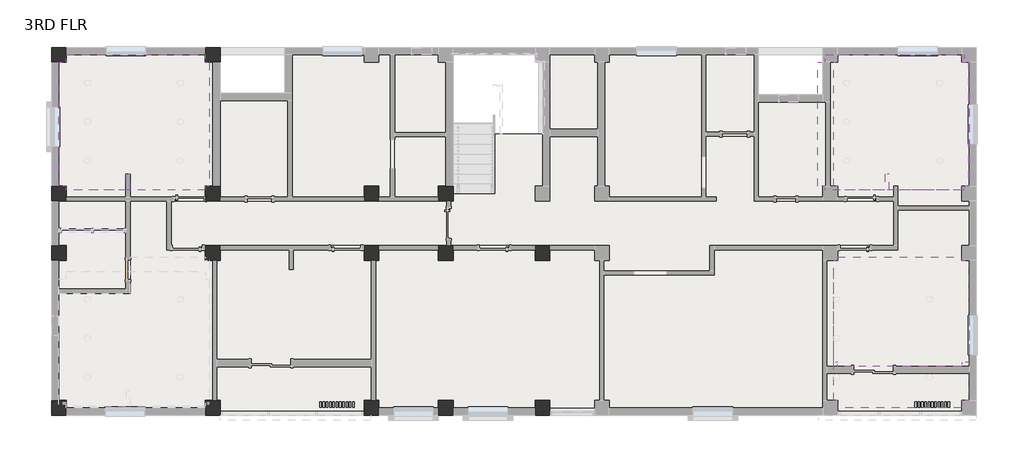
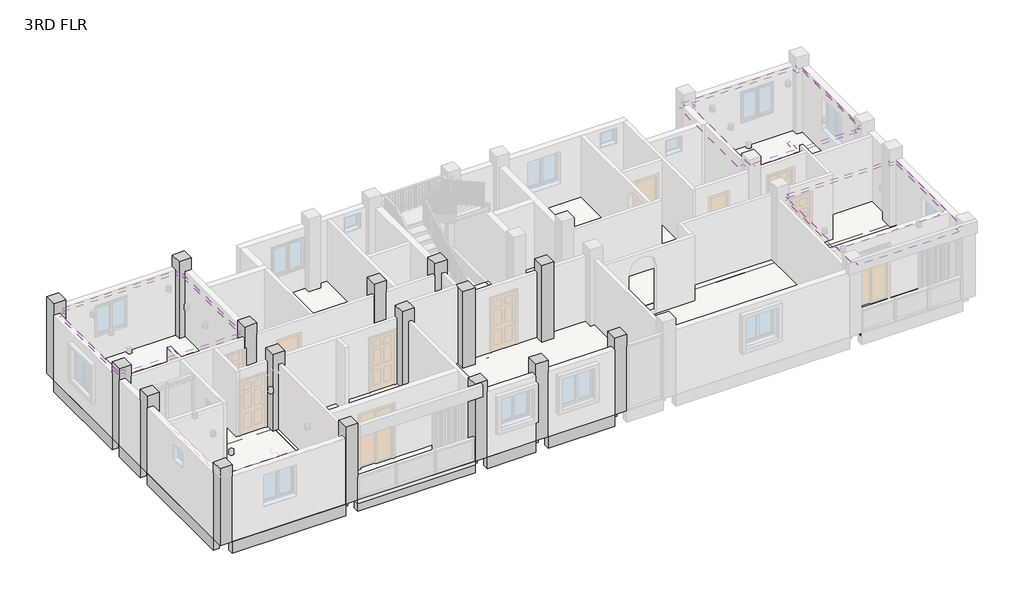
# One storey, part 3 of 5: 23 beams, 16 columns, 6 coverings, 3 slabs.
"""IFC4 building model written with IfcOpenShell, lengths in millimetres."""

from ifc_helpers import new_model, si_unit, point, frame, frame_2d, origin, place, context, project, spatial, polyline, circle_curve, trimmed, segment, composite_curve, outline, extrude, element, save

model = new_model("IFC4")

# Units and contexts
model_context = context("Model", 3, world=origin())
ifc_project = project(units=[si_unit("LENGTHUNIT", "METRE", prefix="MILLI")], contexts=[model_context])

# Site, building, storey
site = spatial("IfcSite", under=ifc_project)
building = spatial("IfcBuilding", under=site)
storey = spatial("IfcBuildingStorey", under=building, Name="3RD FLR", Elevation=9448.8)

# Beams
placement = place(None, origin())
element("IfcBeam", 1, ObjectType="Concrete-Rectangular Beam : 9\" X 18\" BEAM", at=placement, inside=storey, context=model_context, shape_type="SweptSolid", body=[
    extrude(outline(polyline([(-10649.5456086, -10887.8679047), (-10649.5456086, -11116.4679047), (-14916.7456086, -11116.4679047), (-14916.7456086, -10887.8679047), (-10649.5456086, -10887.8679047)])), frame((0.0, 0.0, 8991.6), z_axis=(0.0, 0.0, 1.0), x_axis=(1.0, 0.0, 0.0)), (0.0, 0.0, 1.0), 457.2),
])
element("IfcBeam", 2, ObjectType="Concrete-Rectangular Beam : 9\" X 18\" BEAM", at=placement, inside=storey, context=model_context, shape_type="SweptSolid", body=[
    extrude(outline(polyline([(-5772.7456086, -10887.8679047), (-5772.7456086, -11116.4679047), (-10192.3456086, -11116.4679047), (-10192.3456086, -10887.8679047), (-5772.7456086, -10887.8679047)])), frame((0.0, 0.0, 8991.6), z_axis=(0.0, 0.0, 1.0), x_axis=(1.0, 0.0, 0.0)), (0.0, 0.0, 1.0), 457.2),
])
element("IfcBeam", 3, ObjectType="Concrete-Rectangular Beam : 9\" X 18\" BEAM", at=placement, inside=storey, context=model_context, shape_type="SweptSolid", body=[
    extrude(outline(polyline([(-3486.7456086, -10887.8679047), (-3486.7456086, -11116.4679047), (-5315.5456086, -11116.4679047), (-5315.5456086, -10887.8679047), (-3486.7456086, -10887.8679047)])), frame((0.0, 0.0, 8991.6), z_axis=(0.0, 0.0, 1.0), x_axis=(1.0, 0.0, 0.0)), (0.0, 0.0, 1.0), 457.2),
])
element("IfcBeam", 4, ObjectType="Concrete-Rectangular Beam : 9\" X 18\" BEAM", at=placement, inside=storey, context=model_context, shape_type="SweptSolid", body=[
    extrude(outline(polyline([(-518.4083398, -10887.8679047), (-518.4083398, -11116.4679047), (-3029.5456086, -11116.4679047), (-3029.5456086, -10887.8679047), (-518.4083398, -10887.8679047)])), frame((0.0, 0.0, 8991.6), z_axis=(0.0, 0.0, 1.0), x_axis=(1.0, 0.0, 0.0)), (0.0, 0.0, 1.0), 457.2),
])
element("IfcBeam", 5, ObjectType="Concrete-Rectangular Beam : 9\" X 18\" BEAM", at=placement, inside=storey, context=model_context, shape_type="SweptSolid", body=[
    extrude(outline(polyline([(-15145.3456086, -4072.3794704), (-15373.9456086, -4072.3794704), (-15373.9456086, -262.3794704), (-15145.3456086, -262.3794704), (-15145.3456086, -4072.3794704)])), frame((0.0, 0.0, 8991.6), z_axis=(0.0, 0.0, 1.0), x_axis=(1.0, 0.0, 0.0)), (0.0, 0.0, 1.0), 457.2),
])
element("IfcBeam", 6, ObjectType="Concrete-Rectangular Beam : 9\" X 18\" BEAM", at=placement, inside=storey, context=model_context, shape_type="SweptSolid", body=[
    extrude(outline(polyline([(-15145.3456086, -5901.1794704), (-15373.9456086, -5901.1794704), (-15373.9456086, -4529.5794704), (-15145.3456086, -4529.5794704), (-15145.3456086, -5901.1794704)])), frame((0.0, 0.0, 8991.6), z_axis=(0.0, 0.0, 1.0), x_axis=(1.0, 0.0, 0.0)), (0.0, 0.0, 1.0), 457.2),
])
element("IfcBeam", 7, ObjectType="Concrete-Rectangular Beam : 9\" X 18\" BEAM", at=placement, inside=storey, context=model_context, shape_type="SweptSolid", body=[
    extrude(outline(polyline([(-15145.3456086, -10659.2679047), (-15373.9456086, -10659.2679047), (-15373.9456086, -6358.3794704), (-15145.3456086, -6358.3794704), (-15145.3456086, -10659.2679047)])), frame((0.0, 0.0, 8991.6), z_axis=(0.0, 0.0, 1.0), x_axis=(1.0, 0.0, 0.0)), (0.0, 0.0, 1.0), 457.2),
])
element("IfcBeam", 8, ObjectType="Concrete-Rectangular Beam : 9\" X 18\" BEAM", at=placement, inside=storey, context=model_context, shape_type="SweptSolid", body=[
    extrude(outline(polyline([(-10649.5456086, -4186.6794704), (-10649.5456086, -4415.2794704), (-14916.7456086, -4415.2794704), (-14916.7456086, -4186.6794704), (-10649.5456086, -4186.6794704)])), frame((0.0, 0.0, 8991.6), z_axis=(0.0, 0.0, 1.0), x_axis=(1.0, 0.0, 0.0)), (0.0, 0.0, 1.0), 457.2),
])
element("IfcBeam", 9, ObjectType="Concrete-Rectangular Beam : 9\" X 18\" BEAM", at=placement, inside=storey, context=model_context, shape_type="SweptSolid", body=[
    extrude(outline(polyline([(-5772.7456086, -4186.6794704), (-5772.7456086, -4415.2794704), (-10192.3456086, -4415.2794704), (-10192.3456086, -4186.6794704), (-5772.7456086, -4186.6794704)])), frame((0.0, 0.0, 8991.6), z_axis=(0.0, 0.0, 1.0), x_axis=(1.0, 0.0, 0.0)), (0.0, 0.0, 1.0), 457.2),
])
element("IfcBeam", 10, ObjectType="Concrete-Rectangular Beam : 9\" X 18\" BEAM", at=placement, inside=storey, context=model_context, shape_type="SweptSolid", body=[
    extrude(outline(polyline([(-3486.7456086, -4186.6794704), (-3486.7456086, -4415.2794704), (-5315.5456086, -4415.2794704), (-5315.5456086, -4186.6794704), (-3486.7456086, -4186.6794704)])), frame((0.0, 0.0, 8991.6), z_axis=(0.0, 0.0, 1.0), x_axis=(1.0, 0.0, 0.0)), (0.0, 0.0, 1.0), 457.2),
])
element("IfcBeam", 11, ObjectType="Concrete-Rectangular Beam : 9\" X 18\" BEAM", at=placement, inside=storey, context=model_context, shape_type="SweptSolid", body=[
    extrude(outline(polyline([(-10306.6456086, -4072.3794704), (-10535.2456086, -4072.3794704), (-10535.2456086, -262.3794704), (-10306.6456086, -262.3794704), (-10306.6456086, -4072.3794704)])), frame((0.0, 0.0, 8991.6), z_axis=(0.0, 0.0, 1.0), x_axis=(1.0, 0.0, 0.0)), (0.0, 0.0, 1.0), 457.2),
])
element("IfcBeam", 12, ObjectType="Concrete-Rectangular Beam : 9\" X 18\" BEAM", at=placement, inside=storey, context=model_context, shape_type="SweptSolid", body=[
    extrude(outline(polyline([(-10649.5456086, -6015.4794704), (-10649.5456086, -6244.0794704), (-14916.7456086, -6244.0794704), (-14916.7456086, -6015.4794704), (-10649.5456086, -6015.4794704)])), frame((0.0, 0.0, 8991.6), z_axis=(0.0, 0.0, 1.0), x_axis=(1.0, 0.0, 0.0)), (0.0, 0.0, 1.0), 457.2),
])
element("IfcBeam", 13, ObjectType="Concrete-Rectangular Beam : 9\" X 18\" BEAM", at=placement, inside=storey, context=model_context, shape_type="SweptSolid", body=[
    extrude(outline(polyline([(-5772.7456086, -6015.4794704), (-5772.7456086, -6244.0794704), (-10192.3456086, -6244.0794704), (-10192.3456086, -6015.4794704), (-5772.7456086, -6015.4794704)])), frame((0.0, 0.0, 8991.6), z_axis=(0.0, 0.0, 1.0), x_axis=(1.0, 0.0, 0.0)), (0.0, 0.0, 1.0), 457.2),
])
element("IfcBeam", 14, ObjectType="Concrete-Rectangular Beam : 9\" X 18\" BEAM", at=placement, inside=storey, context=model_context, shape_type="SweptSolid", body=[
    extrude(outline(polyline([(-3486.7456086, -6015.4794704), (-3486.7456086, -6244.0794704), (-5315.5456086, -6244.0794704), (-5315.5456086, -6015.4794704), (-3486.7456086, -6015.4794704)])), frame((0.0, 0.0, 8991.6), z_axis=(0.0, 0.0, 1.0), x_axis=(1.0, 0.0, 0.0)), (0.0, 0.0, 1.0), 457.2),
])
element("IfcBeam", 15, ObjectType="Concrete-Rectangular Beam : 9\" X 18\" BEAM", at=placement, inside=storey, context=model_context, shape_type="SweptSolid", body=[
    extrude(outline(polyline([(-3029.5456086, -6244.0794704), (-3029.5456086, -6015.4794704), (-518.4083398, -6015.4794704), (-518.4083398, -6244.0794704), (-3029.5456086, -6244.0794704)])), frame((0.0, 0.0, 8991.6), z_axis=(0.0, 0.0, 1.0), x_axis=(1.0, 0.0, 0.0)), (0.0, 0.0, 1.0), 457.2),
])
element("IfcBeam", 16, ObjectType="Concrete-Rectangular Beam : 9\" X 18\" BEAM", at=placement, inside=storey, context=model_context, shape_type="SweptSolid", body=[
    extrude(outline(polyline([(-10535.2456086, -6358.3794704), (-10306.6456086, -6358.3794704), (-10306.6456086, -10659.2679047), (-10535.2456086, -10659.2679047), (-10535.2456086, -6358.3794704)])), frame((0.0, 0.0, 8991.6), z_axis=(0.0, 0.0, 1.0), x_axis=(1.0, 0.0, 0.0)), (0.0, 0.0, 1.0), 457.2),
])
element("IfcBeam", 17, ObjectType="Concrete-Rectangular Beam : 9\" X 18\" BEAM", at=placement, inside=storey, context=model_context, shape_type="SweptSolid", body=[
    extrude(outline(polyline([(-5658.4456086, -6358.3794704), (-5429.8456086, -6358.3794704), (-5429.8456086, -10659.2679047), (-5658.4456086, -10659.2679047), (-5658.4456086, -6358.3794704)])), frame((0.0, 0.0, 8991.6), z_axis=(0.0, 0.0, 1.0), x_axis=(1.0, 0.0, 0.0)), (0.0, 0.0, 1.0), 457.2),
])
element("IfcBeam", 18, ObjectType="Concrete-Rectangular Beam : 9\" X 18\" BEAM", at=placement, inside=storey, context=model_context, shape_type="SweptSolid", body=[
    extrude(outline(polyline([(-3372.4456086, -6358.3794704), (-3143.8456086, -6358.3794704), (-3143.8456086, -10659.2679047), (-3372.4456086, -10659.2679047), (-3372.4456086, -6358.3794704)])), frame((0.0, 0.0, 8991.6), z_axis=(0.0, 0.0, 1.0), x_axis=(1.0, 0.0, 0.0)), (0.0, 0.0, 1.0), 457.2),
])
element("IfcBeam", 19, ObjectType="Concrete-Rectangular Beam : 9\" X 18\" BEAM", at=placement, inside=storey, context=model_context, shape_type="SweptSolid", body=[
    extrude(outline(polyline([(-404.1083398, -6358.3794704), (-175.5083398, -6358.3794704), (-175.5083398, -10659.2679047), (-404.1083398, -10659.2679047), (-404.1083398, -6358.3794704)])), frame((0.0, 0.0, 8991.6), z_axis=(0.0, 0.0, 1.0), x_axis=(1.0, 0.0, 0.0)), (0.0, 0.0, 1.0), 457.2),
])
element("IfcBeam", 20, ObjectType="Concrete-Rectangular Beam : 9\" X 18\" BEAM", at=placement, inside=storey, context=model_context, shape_type="SweptSolid", body=[
    extrude(outline(polyline([(-404.1083398, -4529.5794704), (-175.5083398, -4529.5794704), (-175.5083398, -5901.1794704), (-404.1083398, -5901.1794704), (-404.1083398, -4529.5794704)])), frame((0.0, 0.0, 8991.6), z_axis=(0.0, 0.0, 1.0), x_axis=(1.0, 0.0, 0.0)), (0.0, 0.0, 1.0), 457.2),
])
element("IfcBeam", 21, ObjectType="Concrete-Rectangular Beam : 9\" X 18\" BEAM", at=placement, inside=storey, context=model_context, shape_type="SweptSolid", body=[
    extrude(outline(polyline([(-3143.8456086, -5901.1794704), (-3372.4456086, -5901.1794704), (-3372.4456086, -4529.5794704), (-3143.8456086, -4529.5794704), (-3143.8456086, -5901.1794704)])), frame((0.0, 0.0, 8991.6), z_axis=(0.0, 0.0, 1.0), x_axis=(1.0, 0.0, 0.0)), (0.0, 0.0, 1.0), 457.2),
])
element("IfcBeam", 22, ObjectType="Concrete-Rectangular Beam : 9\" X 18\" BEAM", at=placement, inside=storey, context=model_context, shape_type="SweptSolid", body=[
    extrude(outline(polyline([(-5429.8456086, -5901.1794704), (-5658.4456086, -5901.1794704), (-5658.4456086, -4529.5794704), (-5429.8456086, -4529.5794704), (-5429.8456086, -5901.1794704)])), frame((0.0, 0.0, 8991.6), z_axis=(0.0, 0.0, 1.0), x_axis=(1.0, 0.0, 0.0)), (0.0, 0.0, 1.0), 457.2),
])
element("IfcBeam", 23, ObjectType="Concrete-Rectangular Beam : 9\" X 18\" BEAM", at=placement, inside=storey, context=model_context, shape_type="SweptSolid", body=[
    extrude(outline(polyline([(-10306.6456086, -5901.1794704), (-10535.2456086, -5901.1794704), (-10535.2456086, -4529.5794704), (-10306.6456086, -4529.5794704), (-10306.6456086, -5901.1794704)])), frame((0.0, 0.0, 8991.6), z_axis=(0.0, 0.0, 1.0), x_axis=(1.0, 0.0, 0.0)), (0.0, 0.0, 1.0), 457.2),
])

# Columns
element("IfcColumn", 24, ObjectType="Concrete-Rectangular-Column : COLUMN 18\" X 18\"", at=placement, inside=storey, context=model_context, shape_type="SweptSolid", body=[
    extrude(outline(polyline([(-14916.7456086, 194.8205296), (-14916.7456086, -262.3794704), (-15373.9456086, -262.3794704), (-15373.9456086, 194.8205296), (-14916.7456086, 194.8205296)])), frame((0.0, 0.0, 9448.8), z_axis=(0.0, 0.0, 1.0), x_axis=(1.0, 0.0, 0.0)), (0.0, 0.0, 1.0), 3048.0),
])
element("IfcColumn", 25, ObjectType="Concrete-Rectangular-Column : COLUMN 18\" X 18\"", at=placement, inside=storey, context=model_context, shape_type="SweptSolid", body=[
    extrude(outline(polyline([(-10192.3456086, 194.8205296), (-10192.3456086, -262.3794704), (-10649.5456086, -262.3794704), (-10649.5456086, 194.8205296), (-10192.3456086, 194.8205296)])), frame((0.0, 0.0, 9448.8), z_axis=(0.0, 0.0, 1.0), x_axis=(1.0, 0.0, 0.0)), (0.0, 0.0, 1.0), 3048.0),
])
element("IfcColumn", 26, ObjectType="Concrete-Rectangular-Column : COLUMN 18\" X 18\"", at=placement, inside=storey, context=model_context, shape_type="SweptSolid", body=[
    extrude(outline(polyline([(-61.2083398, -10659.2679047), (-61.2083398, -11116.4679047), (-518.4083398, -11116.4679047), (-518.4083398, -10659.2679047), (-61.2083398, -10659.2679047)])), frame((0.0, 0.0, 9448.8), z_axis=(0.0, 0.0, 1.0), x_axis=(1.0, 0.0, 0.0)), (0.0, 0.0, 1.0), 3048.0),
])
element("IfcColumn", 27, ObjectType="Concrete-Rectangular-Column : COLUMN 18\" X 18\"", at=placement, inside=storey, context=model_context, shape_type="SweptSolid", body=[
    extrude(outline(polyline([(-3029.5456086, -10659.2679047), (-3029.5456086, -11116.4679047), (-3486.7456086, -11116.4679047), (-3486.7456086, -10659.2679047), (-3029.5456086, -10659.2679047)])), frame((0.0, 0.0, 9448.8), z_axis=(0.0, 0.0, 1.0), x_axis=(1.0, 0.0, 0.0)), (0.0, 0.0, 1.0), 3048.0),
])
element("IfcColumn", 28, ObjectType="Concrete-Rectangular-Column : COLUMN 18\" X 18\"", at=placement, inside=storey, context=model_context, shape_type="SweptSolid", body=[
    extrude(outline(polyline([(-5315.5456086, -10659.2679047), (-5315.5456086, -11116.4679047), (-5772.7456086, -11116.4679047), (-5772.7456086, -10659.2679047), (-5315.5456086, -10659.2679047)])), frame((0.0, 0.0, 9448.8), z_axis=(0.0, 0.0, 1.0), x_axis=(1.0, 0.0, 0.0)), (0.0, 0.0, 1.0), 3048.0),
])
element("IfcColumn", 29, ObjectType="Concrete-Rectangular-Column : COLUMN 18\" X 18\"", at=placement, inside=storey, context=model_context, shape_type="SweptSolid", body=[
    extrude(outline(polyline([(-10192.3456086, -10659.2679047), (-10192.3456086, -11116.4679047), (-10649.5456086, -11116.4679047), (-10649.5456086, -10659.2679047), (-10192.3456086, -10659.2679047)])), frame((0.0, 0.0, 9448.8), z_axis=(0.0, 0.0, 1.0), x_axis=(1.0, 0.0, 0.0)), (0.0, 0.0, 1.0), 3048.0),
])
element("IfcColumn", 30, ObjectType="Concrete-Rectangular-Column : COLUMN 18\" X 18\"", at=placement, inside=storey, context=model_context, shape_type="SweptSolid", body=[
    extrude(outline(polyline([(-14916.7456086, -10659.2679047), (-14916.7456086, -11116.4679047), (-15373.9456086, -11116.4679047), (-15373.9456086, -10659.2679047), (-14916.7456086, -10659.2679047)])), frame((0.0, 0.0, 9448.8), z_axis=(0.0, 0.0, 1.0), x_axis=(1.0, 0.0, 0.0)), (0.0, 0.0, 1.0), 3048.0),
])
element("IfcColumn", 31, ObjectType="Concrete-Rectangular-Column : COLUMN 18\" X 18\"", at=placement, inside=storey, context=model_context, shape_type="SweptSolid", body=[
    extrude(outline(polyline([(-14916.7456086, -5901.1794704), (-14916.7456086, -6358.3794704), (-15373.9456086, -6358.3794704), (-15373.9456086, -5901.1794704), (-14916.7456086, -5901.1794704)])), frame((0.0, 0.0, 9448.8), z_axis=(0.0, 0.0, 1.0), x_axis=(1.0, 0.0, 0.0)), (0.0, 0.0, 1.0), 3048.0),
])
element("IfcColumn", 32, ObjectType="Concrete-Rectangular-Column : COLUMN 18\" X 18\"", at=placement, inside=storey, context=model_context, shape_type="SweptSolid", body=[
    extrude(outline(polyline([(-14916.7456086, -4072.3794704), (-14916.7456086, -4529.5794704), (-15373.9456086, -4529.5794704), (-15373.9456086, -4072.3794704), (-14916.7456086, -4072.3794704)])), frame((0.0, 0.0, 9448.8), z_axis=(0.0, 0.0, 1.0), x_axis=(1.0, 0.0, 0.0)), (0.0, 0.0, 1.0), 3048.0),
])
element("IfcColumn", 33, ObjectType="Concrete-Rectangular-Column : COLUMN 18\" X 18\"", at=placement, inside=storey, context=model_context, shape_type="SweptSolid", body=[
    extrude(outline(polyline([(-10192.3456086, -4072.3794704), (-10192.3456086, -4529.5794704), (-10649.5456086, -4529.5794704), (-10649.5456086, -4072.3794704), (-10192.3456086, -4072.3794704)])), frame((0.0, 0.0, 9448.8), z_axis=(0.0, 0.0, 1.0), x_axis=(1.0, 0.0, 0.0)), (0.0, 0.0, 1.0), 3048.0),
])
element("IfcColumn", 34, ObjectType="Concrete-Rectangular-Column : COLUMN 18\" X 18\"", at=placement, inside=storey, context=model_context, shape_type="SweptSolid", body=[
    extrude(outline(polyline([(-5315.5456086, -4072.3794704), (-5315.5456086, -4529.5794704), (-5772.7456086, -4529.5794704), (-5772.7456086, -4072.3794704), (-5315.5456086, -4072.3794704)])), frame((0.0, 0.0, 9448.8), z_axis=(0.0, 0.0, 1.0), x_axis=(1.0, 0.0, 0.0)), (0.0, 0.0, 1.0), 3048.0),
])
element("IfcColumn", 35, ObjectType="Concrete-Rectangular-Column : COLUMN 18\" X 18\"", at=placement, inside=storey, context=model_context, shape_type="SweptSolid", body=[
    extrude(outline(polyline([(-3029.5456086, -4072.3794704), (-3029.5456086, -4529.5794704), (-3486.7456086, -4529.5794704), (-3486.7456086, -4072.3794704), (-3029.5456086, -4072.3794704)])), frame((0.0, 0.0, 9448.8), z_axis=(0.0, 0.0, 1.0), x_axis=(1.0, 0.0, 0.0)), (0.0, 0.0, 1.0), 3048.0),
])
element("IfcColumn", 36, ObjectType="Concrete-Rectangular-Column : COLUMN 18\" X 18\"", at=placement, inside=storey, context=model_context, shape_type="SweptSolid", body=[
    extrude(outline(polyline([(-61.2083398, -5901.1794704), (-61.2083398, -6358.3794704), (-518.4083398, -6358.3794704), (-518.4083398, -5901.1794704), (-61.2083398, -5901.1794704)])), frame((0.0, 0.0, 9448.8), z_axis=(0.0, 0.0, 1.0), x_axis=(1.0, 0.0, 0.0)), (0.0, 0.0, 1.0), 3048.0),
])
element("IfcColumn", 37, ObjectType="Concrete-Rectangular-Column : COLUMN 18\" X 18\"", at=placement, inside=storey, context=model_context, shape_type="SweptSolid", body=[
    extrude(outline(polyline([(-3029.5456086, -5901.1794704), (-3029.5456086, -6358.3794704), (-3486.7456086, -6358.3794704), (-3486.7456086, -5901.1794704), (-3029.5456086, -5901.1794704)])), frame((0.0, 0.0, 9448.8), z_axis=(0.0, 0.0, 1.0), x_axis=(1.0, 0.0, 0.0)), (0.0, 0.0, 1.0), 3048.0),
])
element("IfcColumn", 38, ObjectType="Concrete-Rectangular-Column : COLUMN 18\" X 18\"", at=placement, inside=storey, context=model_context, shape_type="SweptSolid", body=[
    extrude(outline(polyline([(-5315.5456086, -5901.1794704), (-5315.5456086, -6358.3794704), (-5772.7456086, -6358.3794704), (-5772.7456086, -5901.1794704), (-5315.5456086, -5901.1794704)])), frame((0.0, 0.0, 9448.8), z_axis=(0.0, 0.0, 1.0), x_axis=(1.0, 0.0, 0.0)), (0.0, 0.0, 1.0), 3048.0),
])
element("IfcColumn", 39, ObjectType="Concrete-Rectangular-Column : COLUMN 18\" X 18\"", at=placement, inside=storey, context=model_context, shape_type="SweptSolid", body=[
    extrude(outline(polyline([(-10192.3456086, -5901.1794704), (-10192.3456086, -6358.3794704), (-10649.5456086, -6358.3794704), (-10649.5456086, -5901.1794704), (-10192.3456086, -5901.1794704)])), frame((0.0, 0.0, 9448.8), z_axis=(0.0, 0.0, 1.0), x_axis=(1.0, 0.0, 0.0)), (0.0, 0.0, 1.0), 3048.0),
])

# Coverings
element("IfcCovering", 40, ObjectType="GWB on Mtl. Stud", at=placement, inside=storey, context=model_context, shape_type="SweptSolid", body=[
    extrude(outline(polyline([(-14916.7456086, -262.3794704), (-14916.7456086, -33.7794704), (-10649.5456086, -33.7794704), (-10649.5456086, -262.3794704), (-10535.2456086, -262.3794704), (-10535.2456086, -4072.3794704), (-10649.5456086, -4072.3794704), (-10649.5456086, -4186.6794704), (-12959.7401855, -4186.6794704), (-12959.7401855, -3705.5659448), (-13086.7401855, -3705.5659448), (-13086.7401855, -4186.6794704), (-14916.7456086, -4186.6794704), (-14916.7456086, -4072.3794704), (-15145.3456086, -4072.3794704), (-15145.3456086, -262.3794704), (-14916.7456086, -262.3794704)]), holes=[composite_curve([segment(trimmed(circle_curve(frame_2d((-14269.0456086, -897.3794704)), 76.2), [point((-14345.2456086, -897.3794704))], [point((-14192.8456086, -897.3794704))], True, "CARTESIAN"), True, "CONTINUOUS"), segment(trimmed(circle_curve(frame_2d((-14269.0456086, -897.3794704)), 76.2), [point((-14192.8456086, -897.3794704))], [point((-14345.2456086, -897.3794704))], True, "CARTESIAN"), True, "CONTINUOUS")], self_intersect=False), composite_curve([segment(trimmed(circle_curve(frame_2d((-14269.0456086, -3284.9794704)), 76.2), [point((-14345.2456086, -3284.9794704))], [point((-14192.8456086, -3284.9794704))], True, "CARTESIAN"), True, "CONTINUOUS"), segment(trimmed(circle_curve(frame_2d((-14269.0456086, -3284.9794704)), 76.2), [point((-14192.8456086, -3284.9794704))], [point((-14345.2456086, -3284.9794704))], True, "CARTESIAN"), True, "CONTINUOUS")], self_intersect=False), composite_curve([segment(trimmed(circle_curve(frame_2d((-14269.0456086, -2091.1794704)), 76.2), [point((-14345.2456086, -2091.1794704))], [point((-14192.8456086, -2091.1794704))], True, "CARTESIAN"), True, "CONTINUOUS"), segment(trimmed(circle_curve(frame_2d((-14269.0456086, -2091.1794704)), 76.2), [point((-14192.8456086, -2091.1794704))], [point((-14345.2456086, -2091.1794704))], True, "CARTESIAN"), True, "CONTINUOUS")], self_intersect=False), composite_curve([segment(trimmed(circle_curve(frame_2d((-11411.5456086, -897.3794704)), 76.2), [point((-11335.3456086, -897.3794704))], [point((-11487.7456086, -897.3794704))], True, "CARTESIAN"), True, "CONTINUOUS"), segment(trimmed(circle_curve(frame_2d((-11411.5456086, -897.3794704)), 76.2), [point((-11487.7456086, -897.3794704))], [point((-11335.3456086, -897.3794704))], True, "CARTESIAN"), True, "CONTINUOUS")], self_intersect=False), composite_curve([segment(trimmed(circle_curve(frame_2d((-11411.5456086, -3284.9794704)), 76.2), [point((-11335.3456086, -3284.9794704))], [point((-11487.7456086, -3284.9794704))], True, "CARTESIAN"), True, "CONTINUOUS"), segment(trimmed(circle_curve(frame_2d((-11411.5456086, -3284.9794704)), 76.2), [point((-11487.7456086, -3284.9794704))], [point((-11335.3456086, -3284.9794704))], True, "CARTESIAN"), True, "CONTINUOUS")], self_intersect=False), composite_curve([segment(trimmed(circle_curve(frame_2d((-11411.5456086, -2091.1794704)), 76.2), [point((-11335.3456086, -2091.1794704))], [point((-11487.7456086, -2091.1794704))], True, "CARTESIAN"), True, "CONTINUOUS"), segment(trimmed(circle_curve(frame_2d((-11411.5456086, -2091.1794704)), 76.2), [point((-11487.7456086, -2091.1794704))], [point((-11335.3456086, -2091.1794704))], True, "CARTESIAN"), True, "CONTINUOUS")], self_intersect=False)]), frame((0.0, 0.0, 12014.2), z_axis=(0.0, 0.0, 1.0), x_axis=(1.0, 0.0, 0.0)), (0.0, 0.0, 1.0), 107.95),
])
element("IfcCovering", 41, ObjectType="GWB on Mtl. Stud", at=placement, inside=storey, context=model_context, shape_type="SweptSolid", body=[
    extrude(outline(polyline([(-15145.3456086, -4072.3794704), (-15145.3456086, -262.3794704), (-14916.7456086, -262.3794704), (-14916.7456086, -33.7794704), (-10649.5456086, -33.7794704), (-10649.5456086, -262.3794704), (-10535.2456086, -262.3794704), (-10535.2456086, -4072.3794704), (-10649.5456086, -4072.3794704), (-10649.5456086, -4186.6794704), (-12959.7401855, -4186.6794704), (-14916.7456086, -4186.6794704), (-14916.7456086, -4072.3794704), (-15145.3456086, -4072.3794704)]), holes=[polyline([(-14840.5456086, -3881.8794704), (-10840.0456086, -3881.8794704), (-10840.0456086, -338.5794704), (-14840.5456086, -338.5794704), (-14840.5456086, -3881.8794704)])]), frame((0.0, 0.0, 11887.2), z_axis=(0.0, 0.0, 1.0), x_axis=(1.0, 0.0, 0.0)), (0.0, 0.0, 1.0), 107.95),
    extrude(outline(polyline([(-14688.1456086, -3729.4794704), (-14688.1456086, -490.9794704), (-10992.4456086, -490.9794704), (-10992.4456086, -3729.4794704), (-14688.1456086, -3729.4794704)]), holes=[polyline([(-11144.8456086, -643.3794704), (-14535.7456086, -643.3794704), (-14535.7456086, -3577.0794704), (-11144.8456086, -3577.0794704), (-11144.8456086, -643.3794704)])]), frame((0.0, 0.0, 11887.2), z_axis=(0.0, 0.0, 1.0), x_axis=(1.0, 0.0, 0.0)), (0.0, 0.0, 1.0), 107.95),
])
element("IfcCovering", 42, ObjectType="GWB on Mtl. Stud", at=placement, inside=storey, context=model_context, shape_type="SweptSolid", body=[
    extrude(outline(polyline([(8991.0043914, -3729.4794704), (8991.0043914, -490.9794704), (12477.1543914, -490.9794704), (12477.1543914, -3729.4794704), (8991.0043914, -3729.4794704)]), holes=[polyline([(12324.7543914, -643.3794704), (9162.4543914, -643.3794704), (9162.4543914, -3577.0794704), (12324.7543914, -3577.0794704), (12324.7543914, -643.3794704)])]), frame((0.0, 0.0, 11887.2), z_axis=(0.0, 0.0, 1.0), x_axis=(1.0, 0.0, 0.0)), (0.0, 0.0, 1.0), 107.95),
    extrude(outline(polyline([(8660.1098601, -4072.3794704), (8660.1098601, -262.3794704), (8774.4128058, -262.3794704), (8774.4128058, -33.7794704), (12584.4128058, -33.7794704), (12584.4128058, -262.3794704), (12813.0098601, -262.3794704), (12813.0098601, -4072.3794704), (12584.4128058, -4072.3794704), (12584.4128058, -4186.6794704), (10509.8598145, -4186.6794704), (8774.4128058, -4186.6794704), (8774.4128058, -4072.3794704), (8660.1098601, -4072.3794704)]), holes=[polyline([(8838.6043914, -338.5794704), (8838.6043914, -3881.8794704), (12629.5543914, -3881.8794704), (12629.5543914, -338.5794704), (8838.6043914, -338.5794704)])]), frame((0.0, 0.0, 11887.2), z_axis=(0.0, 0.0, 1.0), x_axis=(1.0, 0.0, 0.0)), (0.0, 0.0, 1.0), 107.95),
])
element("IfcCovering", 43, ObjectType="GWB on Mtl. Stud", at=placement, inside=storey, context=model_context, shape_type="SweptSolid", body=[
    extrude(outline(polyline([(8991.0043914, -9147.9642361), (8991.0043914, -6726.6794704), (12477.1543914, -6726.6794704), (12477.1543914, -9147.9642361), (8991.0043914, -9147.9642361)]), holes=[polyline([(12324.7543914, -7031.4298611), (9162.4543914, -7031.4298611), (9162.4543914, -8995.5642361), (12324.7543914, -8995.5642361), (12324.7543914, -7031.4298611)])]), frame((0.0, 0.0, 11887.2), z_axis=(0.0, 0.0, 1.0), x_axis=(1.0, 0.0, 0.0)), (0.0, 0.0, 1.0), 107.95),
    extrude(outline(polyline([(8660.1098601, -9490.8642361), (8660.1098601, -6358.3685356), (8774.4128058, -6358.3685356), (8774.4128058, -6244.0794704), (12584.4128058, -6244.0794704), (12584.4128058, -6358.3794704), (12813.0098601, -6358.3794704), (12813.0098601, -9490.8642361), (12584.4128058, -9490.8642361), (12584.4128058, -9605.1642361), (10509.8598145, -9605.1642361), (8774.4128058, -9605.1642361), (8774.4128058, -9490.8642361), (8660.1098601, -9490.8642361)]), holes=[polyline([(12629.5543914, -6498.0794704), (8838.6043914, -6498.0794704), (8838.6043914, -9300.3642361), (12629.5543914, -9300.3642361), (12629.5543914, -6498.0794704)])]), frame((0.0, 0.0, 11887.2), z_axis=(0.0, 0.0, 1.0), x_axis=(1.0, 0.0, 0.0)), (0.0, 0.0, 1.0), 107.95),
])
element("IfcCovering", 44, ObjectType="GWB on Mtl. Stud", at=placement, inside=storey, context=model_context, shape_type="SweptSolid", body=[
    extrude(outline(polyline([(8400.4543914, -262.3794704), (8400.4543914, -33.7794704), (12667.6543914, -33.7794704), (12667.6543914, -262.3794704), (12781.9543914, -262.3794704), (12781.9543914, -4072.3794704), (12667.6543914, -4072.3794704), (12667.6543914, -4186.6794704), (10357.4598145, -4186.6794704), (10357.4598145, -3705.5659448), (10230.4598145, -3705.5659448), (10230.4598145, -4186.6794704), (8400.4543914, -4186.6794704), (8400.4543914, -4072.3794704), (8171.8543914, -4072.3794704), (8171.8543914, -262.3794704), (8400.4543914, -262.3794704)]), holes=[composite_curve([segment(trimmed(circle_curve(frame_2d((9048.1543914, -897.3794704)), 76.2), [point((8971.9543914, -897.3794704))], [point((9124.3543914, -897.3794704))], True, "CARTESIAN"), True, "CONTINUOUS"), segment(trimmed(circle_curve(frame_2d((9048.1543914, -897.3794704)), 76.2), [point((9124.3543914, -897.3794704))], [point((8971.9543914, -897.3794704))], True, "CARTESIAN"), True, "CONTINUOUS")], self_intersect=False), composite_curve([segment(trimmed(circle_curve(frame_2d((9048.1543914, -3284.9794704)), 76.2), [point((8971.9543914, -3284.9794704))], [point((9124.3543914, -3284.9794704))], True, "CARTESIAN"), True, "CONTINUOUS"), segment(trimmed(circle_curve(frame_2d((9048.1543914, -3284.9794704)), 76.2), [point((9124.3543914, -3284.9794704))], [point((8971.9543914, -3284.9794704))], True, "CARTESIAN"), True, "CONTINUOUS")], self_intersect=False), composite_curve([segment(trimmed(circle_curve(frame_2d((9048.1543914, -2091.1794704)), 76.2), [point((8971.9543914, -2091.1794704))], [point((9124.3543914, -2091.1794704))], True, "CARTESIAN"), True, "CONTINUOUS"), segment(trimmed(circle_curve(frame_2d((9048.1543914, -2091.1794704)), 76.2), [point((9124.3543914, -2091.1794704))], [point((8971.9543914, -2091.1794704))], True, "CARTESIAN"), True, "CONTINUOUS")], self_intersect=False), composite_curve([segment(trimmed(circle_curve(frame_2d((11905.6543914, -897.3794704)), 76.2), [point((11981.8543914, -897.3794704))], [point((11829.4543914, -897.3794704))], True, "CARTESIAN"), True, "CONTINUOUS"), segment(trimmed(circle_curve(frame_2d((11905.6543914, -897.3794704)), 76.2), [point((11829.4543914, -897.3794704))], [point((11981.8543914, -897.3794704))], True, "CARTESIAN"), True, "CONTINUOUS")], self_intersect=False), composite_curve([segment(trimmed(circle_curve(frame_2d((11905.6543914, -3284.9794704)), 76.2), [point((11981.8543914, -3284.9794704))], [point((11829.4543914, -3284.9794704))], True, "CARTESIAN"), True, "CONTINUOUS"), segment(trimmed(circle_curve(frame_2d((11905.6543914, -3284.9794704)), 76.2), [point((11829.4543914, -3284.9794704))], [point((11981.8543914, -3284.9794704))], True, "CARTESIAN"), True, "CONTINUOUS")], self_intersect=False)]), frame((0.0, 0.0, 12014.2), z_axis=(0.0, 0.0, 1.0), x_axis=(1.0, 0.0, 0.0)), (0.0, 0.0, 1.0), 107.95),
])
element("IfcCovering", 45, ObjectType="GWB on Mtl. Stud", at=placement, inside=storey, context=model_context, shape_type="SweptSolid", body=[
    extrude(outline(polyline([(8660.8043914, -6917.1794704), (8660.8043914, -6358.3794704), (8774.4128058, -6358.3794704), (8774.4128058, -6244.0794704), (12584.4128058, -6244.0794704), (12584.4128058, -6358.3794704), (12813.0098601, -6358.3794704), (12813.0098601, -10659.2679047), (12584.4128058, -10659.2679047), (12584.4128058, -10887.8673366), (8774.4128058, -10887.8673366), (8774.4128058, -10659.2679047), (8660.8043914, -10659.2679047), (8660.8043914, -6917.1794704)]), holes=[composite_curve([segment(trimmed(circle_curve(frame_2d((8743.3543914, -7552.1794704)), 76.2), [point((8667.1543914, -7552.1794704))], [point((8819.5543914, -7552.1794704))], True, "CARTESIAN"), True, "CONTINUOUS"), segment(trimmed(circle_curve(frame_2d((8743.3543914, -7552.1794704)), 76.2), [point((8819.5543914, -7552.1794704))], [point((8667.1543914, -7552.1794704))], True, "CARTESIAN"), True, "CONTINUOUS")], self_intersect=False), composite_curve([segment(trimmed(circle_curve(frame_2d((8743.3543914, -9939.7794704)), 76.2), [point((8667.1543914, -9939.7794704))], [point((8819.5543914, -9939.7794704))], True, "CARTESIAN"), True, "CONTINUOUS"), segment(trimmed(circle_curve(frame_2d((8743.3543914, -9939.7794704)), 76.2), [point((8819.5543914, -9939.7794704))], [point((8667.1543914, -9939.7794704))], True, "CARTESIAN"), True, "CONTINUOUS")], self_intersect=False), composite_curve([segment(trimmed(circle_curve(frame_2d((8743.3543914, -8745.9794704)), 76.2), [point((8667.1543914, -8745.9794704))], [point((8819.5543914, -8745.9794704))], True, "CARTESIAN"), True, "CONTINUOUS"), segment(trimmed(circle_curve(frame_2d((8743.3543914, -8745.9794704)), 76.2), [point((8819.5543914, -8745.9794704))], [point((8667.1543914, -8745.9794704))], True, "CARTESIAN"), True, "CONTINUOUS")], self_intersect=False), composite_curve([segment(trimmed(circle_curve(frame_2d((11600.8543914, -7552.1794704)), 76.2), [point((11677.0543914, -7552.1794704))], [point((11524.6543914, -7552.1794704))], True, "CARTESIAN"), True, "CONTINUOUS"), segment(trimmed(circle_curve(frame_2d((11600.8543914, -7552.1794704)), 76.2), [point((11524.6543914, -7552.1794704))], [point((11677.0543914, -7552.1794704))], True, "CARTESIAN"), True, "CONTINUOUS")], self_intersect=False), composite_curve([segment(trimmed(circle_curve(frame_2d((11600.8543914, -9939.7794704)), 76.2), [point((11677.0543914, -9939.7794704))], [point((11524.6543914, -9939.7794704))], True, "CARTESIAN"), True, "CONTINUOUS"), segment(trimmed(circle_curve(frame_2d((11600.8543914, -9939.7794704)), 76.2), [point((11524.6543914, -9939.7794704))], [point((11677.0543914, -9939.7794704))], True, "CARTESIAN"), True, "CONTINUOUS")], self_intersect=False)]), frame((0.0, 0.0, 12014.2), z_axis=(0.0, 0.0, 1.0), x_axis=(1.0, 0.0, 0.0)), (0.0, 0.0, 1.0), 107.95),
])

# Slabs
element("IfcSlab", 46, ObjectType="white MARBLE FLOORING 6\" 2", at=placement, inside=storey, context=model_context, shape_type="SweptSolid", body=[
    extrude(outline(polyline([(-14916.7456086, -262.3794704), (-14916.7456086, -33.7794704), (-10649.5456086, -33.7794704), (-10649.5456086, -262.3794704), (-10420.9456086, -262.3794704), (-10420.9456086, -4072.3794704), (-10649.5456086, -4072.3794704), (-10649.5456086, -4529.5794704), (-11614.7456086, -4529.5794704), (-11614.7456086, -4402.5794704), (-12959.7401855, -4402.5794704), (-12959.7401855, -3705.5659448), (-13086.7401855, -3705.5659448), (-13086.7401855, -4402.5794704), (-14916.7456086, -4402.5794704), (-14916.7456086, -4072.3794704), (-15145.3456086, -4072.3794704), (-15145.3456086, -262.3794704), (-14916.7456086, -262.3794704)])), frame((0.0, 0.0, 9296.4), z_axis=(0.0, 0.0, 1.0), x_axis=(1.0, 0.0, 0.0)), (0.0, 0.0, 1.0), 152.4),
    extrude(outline(polyline([(-15145.3456086, -7363.1659448), (-12959.7401855, -7363.1659448), (-12959.7401855, -4529.5794704), (-11829.4401855, -4529.5794704), (-11829.4401855, -6028.1794704), (-10649.5456086, -6028.1794704), (-10649.5456086, -6358.3794704), (-10420.9456086, -6358.3794704), (-10420.9456086, -10659.2679047), (-10649.5456086, -10659.2679047), (-10649.5456086, -10887.8679047), (-14916.7456086, -10887.8679047), (-14916.7456086, -10659.2679047), (-15145.3456086, -10659.2679047), (-15145.3456086, -7363.1659448)])), frame((0.0, 0.0, 9296.4), z_axis=(0.0, 0.0, 1.0), x_axis=(1.0, 0.0, 0.0)), (0.0, 0.0, 1.0), 152.4),
    extrude(outline(polyline([(-5772.7456086, -11116.4679047), (-10192.3456086, -11116.4679047), (-10192.3456086, -10659.2679047), (-10293.9456086, -10659.2679047), (-10293.9456086, -9630.5679047), (-9239.8456086, -9630.5679047), (-9239.8456086, -9401.9679047), (-10293.9456086, -9401.9679047), (-10293.9456086, -6358.3794704), (-10192.3456086, -6358.3794704), (-10192.3456086, -6028.1794704), (-8071.4456086, -6028.1794704), (-8071.4456086, -6637.7794704), (-7944.4456086, -6637.7794704), (-7944.4456086, -6028.1794704), (-6788.7456086, -6028.1794704), (-6788.7456086, -5901.1794704), (-5874.3456086, -5901.1794704), (-5874.3456086, -6028.1794704), (-5772.7456086, -6028.1794704), (-5772.7456086, -6358.3794704), (-5544.1456086, -6358.3794704), (-5544.1456086, -9401.9679047), (-8020.6456086, -9401.9679047), (-8020.6456086, -9630.5679047), (-5544.1456086, -9630.5679047), (-5544.1456086, -10659.2679047), (-5772.7456086, -10659.2679047), (-5772.7456086, -11116.4679047)])), frame((0.0, 0.0, 9296.4), z_axis=(0.0, 0.0, 1.0), x_axis=(1.0, 0.0, 0.0)), (0.0, 0.0, 1.0), 152.4),
    extrude(outline(polyline([(-5315.5456086, -10659.2679047), (-5417.1456086, -10659.2679047), (-5417.1456086, -6358.3794704), (-5315.5456086, -6358.3794704), (-5315.5456086, -6028.1794704), (-3486.7456086, -6028.1794704), (-3486.7456086, -6358.3794704), (-3029.5456086, -6358.3794704), (-3029.5456086, -6028.1794704), (-2231.1769742, -6028.1794704), (-2231.1769742, -5901.1794704), (-1316.7769742, -5901.1794704), (-1316.7769742, -6028.1794704), (-518.4083398, -6028.1794704), (-518.4083398, -6358.3794704), (-61.2083398, -6358.3794704), (-61.2083398, -6028.1794704), (1310.3916602, -6028.1794704), (1310.3916602, -6358.3794704), (1462.7916602, -6358.3794704), (1462.7916602, -10659.2679047), (1310.3916602, -10659.2679047), (1310.3916602, -10887.8679047), (-61.2083398, -10887.8679047), (-61.2083398, -10659.2679047), (-518.4083398, -10659.2679047), (-518.4083398, -10887.8679047), (-3029.5456086, -10887.8679047), (-3029.5456086, -10659.2679047), (-3486.7456086, -10659.2679047), (-3486.7456086, -10887.8679047), (-5315.5456086, -10887.8679047), (-5315.5456086, -10659.2679047)])), frame((0.0, 0.0, 9296.4), z_axis=(0.0, 0.0, 1.0), x_axis=(1.0, 0.0, 0.0)), (0.0, 0.0, 1.0), 152.4),
    extrude(outline(polyline([(1589.7916602, -6802.8794704), (4980.6916602, -6802.8794704), (4980.6916602, -6028.1794704), (8317.2128058, -6028.1794704), (8317.2128058, -10887.8679047), (1767.5916602, -10887.8679047), (1767.5916602, -10659.2679047), (1589.7916602, -10659.2679047), (1589.7916602, -6802.8794704)])), frame((0.0, 0.0, 9296.4), z_axis=(0.0, 0.0, 1.0), x_axis=(1.0, 0.0, 0.0)), (0.0, 0.0, 1.0), 152.4),
    extrude(outline(polyline([(8774.4128058, -10659.2679047), (8444.2128058, -10659.2679047), (8444.2128058, -9833.7679047), (9269.7128058, -9833.7679047), (9269.7128058, -9605.1679047), (8444.2128058, -9605.1679047), (8444.2128058, -6358.3794704), (8774.4128058, -6358.3794704), (8774.4128058, -6028.1794704), (8850.6128058, -6028.1794704), (8850.6128058, -5901.1794704), (9765.0128058, -5901.1794704), (9765.0128058, -6028.1794704), (9790.4128058, -6028.1794704), (10628.6128058, -6028.1794704), (10628.6128058, -4808.9794704), (12813.0128058, -4808.9794704), (12813.0128058, -5901.1794704), (12584.4128058, -5901.1794704), (12584.4128058, -6358.3794704), (12813.0128058, -6358.3794704), (12813.0128058, -9605.1679047), (10488.9128058, -9605.1679047), (10488.9128058, -9833.7679047), (12813.0128058, -9833.7679047), (12813.0128058, -10659.2679047), (12584.4128058, -10659.2679047), (12584.4128058, -11052.9679047), (8774.4128058, -11052.9679047), (8774.4128058, -10659.2679047)])), frame((0.0, 0.0, 9296.4), z_axis=(0.0, 0.0, 1.0), x_axis=(1.0, 0.0, 0.0)), (0.0, 0.0, 1.0), 152.4),
    extrude(outline(polyline([(9968.2128058, -4529.5794704), (9053.8128058, -4529.5794704), (8774.4128058, -4529.5794704), (8774.4128058, -4072.3794704), (8545.8128058, -4072.3794704), (8545.8128058, -262.3794704), (8774.4128058, -262.3794704), (8774.4128058, -33.7794704), (12584.4128058, -33.7794704), (12584.4128058, -262.3794704), (12813.0128058, -262.3794704), (12813.0128058, -4072.3794704), (12584.4128058, -4072.3794704), (12584.4128058, -4529.5794704), (12813.0128058, -4529.5794704), (12813.0128058, -4681.9794704), (10628.6128058, -4681.9794704), (10628.6128058, -4072.3794704), (10501.6128058, -4072.3794704), (10501.6128058, -4402.5794704), (9968.2128058, -4402.5794704), (9968.2128058, -4529.5794704)])), frame((0.0, 0.0, 9296.4), z_axis=(0.0, 0.0, 1.0), x_axis=(1.0, 0.0, 0.0)), (0.0, 0.0, 1.0), 152.4),
])
element("IfcSlab", 47, ObjectType="white MARBLE FLOORING 6\" 2", at=placement, inside=storey, context=model_context, shape_type="SweptSolid", body=[
    extrude(outline(polyline([(-11702.4401855, -5901.1794704), (-11702.4401855, -4529.5794704), (-8604.8456086, -4529.5794704), (-3232.7456086, -4529.5794704), (-3232.7456086, -4758.1794704), (-3105.7456086, -4758.1794704), (-3105.7456086, -4529.5794704), (-3029.5456086, -4529.5794704), (-3029.5456086, -4300.9794704), (-1759.5456086, -4300.9794704), (-1759.5456086, -2472.1794704), (-289.8083398, -2472.1794704), (-289.8083398, -4072.3794704), (-518.4083398, -4072.3794704), (-518.4083398, -4529.5794704), (-61.2083398, -4529.5794704), (-61.2083398, -2548.3794704), (1399.2916602, -2548.3794704), (1399.2916602, -4072.3794704), (1310.3916602, -4072.3794704), (1310.3916602, -4529.5794704), (5044.1916602, -4529.5794704), (5044.1916602, -4402.5794704), (4726.6916602, -4402.5794704), (4726.6916602, -2535.6794704), (6212.5916602, -2535.6794704), (6212.5916602, -4529.5794704), (10501.6128058, -4529.5794704), (10501.6128058, -5901.1794704), (4853.6916602, -5901.1794704), (4853.6916602, -6675.8794704), (1589.7916602, -6675.8794704), (1589.7916602, -6358.3794704), (1767.5916602, -6358.3794704), (1767.5916602, -5901.1794704), (-3105.7456086, -5901.1794704), (-3105.7456086, -5672.5794704), (-3232.7456086, -5672.5794704), (-3232.7456086, -5901.1794704), (-10750.542897, -5901.1794704), (-10750.542897, -6028.1794704), (-11664.942897, -6028.1794704), (-11664.942897, -5901.1794704), (-11702.4401855, -5901.1794704)])), frame((0.0, 0.0, 9296.4), z_axis=(0.0, 0.0, 1.0), x_axis=(1.0, 0.0, 0.0)), (0.0, 0.0, 1.0), 152.4),
])
element("IfcSlab", 48, ObjectType="white MARBLE FLOORING 6\" 2", at=placement, inside=storey, context=model_context, shape_type="SweptSolid", body=[
    extrude(outline(polyline([(-61.2083398, -2319.7794704), (-61.2083398, -33.7794704), (1310.3916602, -33.7794704), (1310.3916602, -262.3794704), (1399.2916602, -262.3794704), (1399.2916602, -2319.7794704), (-61.2083398, -2319.7794704)])), frame((0.0, 0.0, 9448.8), z_axis=(0.0, 0.0, 1.0), x_axis=(1.0, 0.0, 0.0)), (0.0, 0.0, 1.0), 152.4),
    extrude(outline(polyline([(1767.5916602, -4072.3794704), (1627.8916602, -4072.3794704), (1627.8916602, -262.3794704), (1767.5916602, -262.3794704), (1767.5916602, -33.7794704), (4599.6916602, -33.7794704), (4599.6916602, -4402.5794704), (1767.5916602, -4402.5794704), (1767.5916602, -4072.3794704)])), frame((0.0, 0.0, 9448.8), z_axis=(0.0, 0.0, 1.0), x_axis=(1.0, 0.0, 0.0)), (0.0, 0.0, 1.0), 152.4),
    extrude(outline(polyline([(6212.5916602, -33.7794704), (6212.5916602, -2408.6794704), (5996.6916602, -2408.6794704), (5996.6916602, -2535.6794704), (5234.6916602, -2535.6794704), (5234.6916602, -2408.6794704), (4726.6916602, -2408.6794704), (4726.6916602, -33.7794704), (6212.5916602, -33.7794704)])), frame((0.0, 0.0, 9448.8), z_axis=(0.0, 0.0, 1.0), x_axis=(1.0, 0.0, 0.0)), (0.0, 0.0, 1.0), 152.4),
    extrude(outline(polyline([(6885.6916602, -4402.5794704), (6339.5916602, -4402.5794704), (6339.5916602, -1481.5794704), (8418.8128058, -1481.5794704), (8418.8128058, -4072.3794704), (8317.2128058, -4072.3794704), (8317.2128058, -4402.5794704), (7495.2916602, -4402.5794704), (7495.2916602, -4529.5794704), (6885.6916602, -4529.5794704), (6885.6916602, -4402.5794704)])), frame((0.0, 0.0, 9448.8), z_axis=(0.0, 0.0, 1.0), x_axis=(1.0, 0.0, 0.0)), (0.0, 0.0, 1.0), 152.4),
    extrude(outline(polyline([(-3486.7456086, -4402.5794704), (-4832.9456086, -4402.5794704), (-4832.9456086, -2548.3794704), (-3258.1456086, -2548.3794704), (-3258.1456086, -4072.3794704), (-3486.7456086, -4072.3794704), (-3486.7456086, -4402.5794704)])), frame((0.0, 0.0, 9448.8), z_axis=(0.0, 0.0, 1.0), x_axis=(1.0, 0.0, 0.0)), (0.0, 0.0, 1.0), 152.4),
    extrude(outline(polyline([(-10192.3456086, -4402.5794704), (-10192.3456086, -1443.4794704), (-8109.5456086, -1443.4794704), (-8109.5456086, -4402.5794704), (-8604.8456086, -4402.5794704), (-8604.8456086, -4529.5794704), (-9366.8456086, -4529.5794704), (-9366.8456086, -4402.5794704), (-10192.3456086, -4402.5794704)])), frame((0.0, 0.0, 9448.8), z_axis=(0.0, 0.0, 1.0), x_axis=(1.0, 0.0, 0.0)), (0.0, 0.0, 1.0), 152.4),
    extrude(outline(polyline([(-4832.9456086, -2421.3794704), (-4832.9456086, -33.7794704), (-3486.7456086, -33.7794704), (-3486.7456086, -262.3794704), (-3258.1456086, -262.3794704), (-3258.1456086, -2421.3794704), (-4832.9456086, -2421.3794704)])), frame((0.0, 0.0, 9448.8), z_axis=(0.0, 0.0, 1.0), x_axis=(1.0, 0.0, 0.0)), (0.0, 0.0, 1.0), 152.4),
    extrude(outline(polyline([(-7982.5456086, -4402.5794704), (-7982.5456086, -33.7794704), (-5772.7456086, -33.7794704), (-5772.7456086, -262.3794704), (-5315.5456086, -262.3794704), (-5315.5456086, -33.7794704), (-4959.9456086, -33.7794704), (-4959.9456086, -4402.5794704), (-5315.5456086, -4402.5794704), (-5315.5456086, -4072.3794704), (-5772.7456086, -4072.3794704), (-5772.7456086, -4402.5794704), (-7982.5456086, -4402.5794704)])), frame((0.0, 0.0, 9448.8), z_axis=(0.0, 0.0, 1.0), x_axis=(1.0, 0.0, 0.0)), (0.0, 0.0, 1.0), 152.4),
    extrude(outline(polyline([(-15145.3456086, -5901.1794704), (-15145.3456086, -4529.5794704), (-13086.7401855, -4529.5794704), (-13086.7401855, -6334.4659448), (-12959.7401855, -6334.4659448), (-12959.7401855, -6944.0659448), (-13086.7401855, -6945.7574008), (-13086.7401855, -7236.1659448), (-15145.3456086, -7236.1659448), (-15145.3456086, -6358.3794704), (-14916.7456086, -6358.3794704), (-14916.7456086, -5901.1794704), (-15145.3456086, -5901.1794704)])), frame((0.0, 0.0, 9448.8), z_axis=(0.0, 0.0, 1.0), x_axis=(1.0, 0.0, 0.0)), (0.0, 0.0, 1.0), 152.4),
])

save(model, "model.ifc")

# Revit data of these elements
# Type "Concrete-Rectangular Beam : 9\" X 18\" BEAM"
#   Assembly Code = "B10"
#   Length [instance default] = 5' - 0"
#   b = 0' - 9"
#   h = 1' - 6"
#   Structural Material [instance default] = Concrete, Cast-in-Place gray
# Type "Concrete-Rectangular-Column : COLUMN 18\" X 18\""
#   Assembly Code = "B10"
#   b = 1' - 6"
#   h = 1' - 6"
#   Structural Material [instance default] = Concrete, Cast-in-Place gray
# Type "GWB on Mtl. Stud"
#   Assembly Code = "C3030220"
#   built-in parameter 1002203 = 1 (stored number, unit not read)
#   built-in parameter 1002202 = 1 (stored number, unit not read)
#   Layers, outside or top first: 0' - 3 5/8" "WHITE CEILING 6\"" (function 1); 0' - 0 5/8" "WHITE CEILING 6\"" (function 5)
# Type "white MARBLE FLOORING 6\" 2"
#   Assembly Code = "B1010"
#   Function = 0
#   Layers, outside or top first: 0' - 6" "MARBLE FLOORING 6\"" (function 1)
# Elements 1, 2, 3, 4, 5, 6, 7 (IfcBeam, "Concrete-Rectangular Beam : 9\" X 18\" BEAM")
#   Structural Material = Concrete, Cast-in-Place gray
#   Phase Created = New Construction
#   Materials on its faces: "Concrete, Cast-in-Place gray", "SAND BEIGE PAINT"
# Elements 8, 9, 10, 11, 12, 13, 14, 15, 16, 17, 18, 19, 20, 21, 22, 23 (IfcBeam, "Concrete-Rectangular Beam : 9\" X 18\" BEAM")
#   Structural Material = Concrete, Cast-in-Place gray
#   Phase Created = New Construction
#   Materials on its faces: "Concrete, Cast-in-Place gray"
# Elements 24, 25, 26, 27, 28, 29, 30, 31, 32 (IfcColumn, "Concrete-Rectangular-Column : COLUMN 18\" X 18\"")
#   Structural Material = Concrete, Cast-in-Place gray
#   Phase Created = New Construction
#   Materials on its faces: "Concrete, Cast-in-Place gray", "SAND BEIGE PAINT"
# Elements 33, 34, 35, 36, 37, 38, 39 (IfcColumn, "Concrete-Rectangular-Column : COLUMN 18\" X 18\"")
#   Structural Material = Concrete, Cast-in-Place gray
#   Phase Created = New Construction
#   Materials on its faces: "Concrete, Cast-in-Place gray"
# Elements 40, 44, 45 (IfcCovering, "GWB on Mtl. Stud")
#   Height Offset From Level = 8' - 5"
#   Phase Created = New Construction
#   Materials on its faces: "WHITE CEILING 6\""
# Elements 41, 42, 43 (IfcCovering, "GWB on Mtl. Stud")
#   Height Offset From Level = 8' - 0"
#   Phase Created = New Construction
#   Materials on its faces: "WHITE CEILING 6\""
# Element 46 (IfcSlab, "white MARBLE FLOORING 6\" 2")
#   Height Offset From Level = 0' - 0"
#   Phase Created = New Construction
#   Materials on its faces: "MARBLE FLOORING 6\""
# Element 47 (IfcSlab, "white MARBLE FLOORING 6\" 2")
#   built-in parameter 1001955 = -1.5708 (stored number, unit not read)
#   Height Offset From Level = 0' - 0"
#   Phase Created = New Construction
#   Materials on its faces: "MARBLE FLOORING 6\""
# Element 48 (IfcSlab, "white MARBLE FLOORING 6\" 2")
#   built-in parameter 1001955 = -1.5708 (stored number, unit not read)
#   Height Offset From Level = 0' - 6"
#   Phase Created = New Construction
#   Materials on its faces: "MARBLE FLOORING 6\""
# Materials
#   "Concrete, Cast-in-Place gray": class "Concrete", colour RGB 192 192 192, transparency 0, Description = "Cast-in-place concrete", Cost = 0
#   "WHITE CEILING 6\"": class "Generic", colour RGB 120 120 120, transparency 0, Cost = 0
#   "MARBLE FLOORING 6\"": class "Generic", colour RGB 120 120 120, transparency 0, Cost = 0
#   "SAND BEIGE PAINT": class "Generic", colour RGB 120 120 120, transparency 0, Cost = 0
